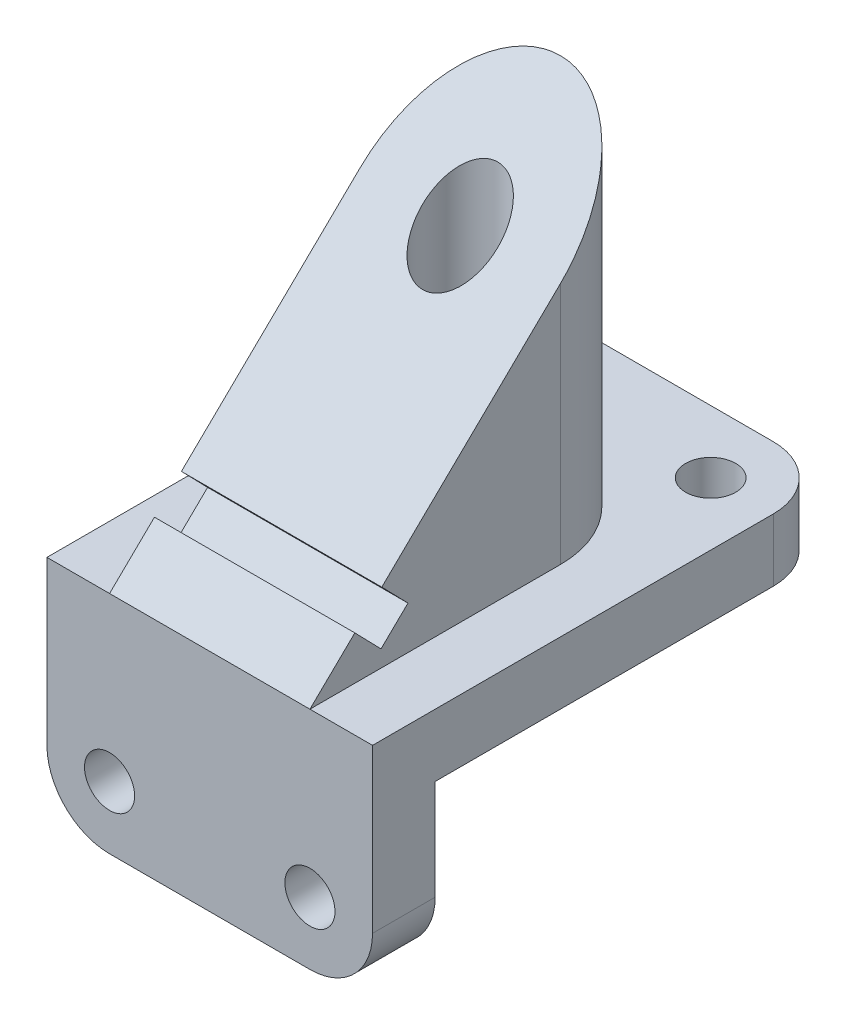
ISO-10303-21;
HEADER;
FILE_DESCRIPTION(('STEP AP214'),'2;1');
FILE_NAME('part.step','',(''),(''),'','','');
FILE_SCHEMA(('AUTOMOTIVE_DESIGN { 1 0 10303 214 1 1 1 1 }'));
ENDSEC;
DATA;
#1=APPLICATION_CONTEXT('core data for automotive mechanical design processes');
#2=APPLICATION_PROTOCOL_DEFINITION('international standard','automotive_design',2000,#1);
#3=PRODUCT_CONTEXT('',#1,'mechanical');
#4=PRODUCT('Part','Part','',(#3));
#5=PRODUCT_RELATED_PRODUCT_CATEGORY('part','',(#4));
#6=PRODUCT_DEFINITION_FORMATION('','',#4);
#7=PRODUCT_DEFINITION_CONTEXT('part definition',#1,'design');
#8=PRODUCT_DEFINITION('design','',#6,#7);
#9=PRODUCT_DEFINITION_SHAPE('','',#8);
#10=(LENGTH_UNIT() NAMED_UNIT(*) SI_UNIT(.MILLI.,.METRE.));
#11=(NAMED_UNIT(*) PLANE_ANGLE_UNIT() SI_UNIT($,.RADIAN.));
#12=(NAMED_UNIT(*) SI_UNIT($,.STERADIAN.) SOLID_ANGLE_UNIT());
#13=UNCERTAINTY_MEASURE_WITH_UNIT(LENGTH_MEASURE(1.E-05),#10,'distance_accuracy_value','');
#14=(GEOMETRIC_REPRESENTATION_CONTEXT(3) GLOBAL_UNCERTAINTY_ASSIGNED_CONTEXT((#13)) GLOBAL_UNIT_ASSIGNED_CONTEXT((#10,
#11,#12)) REPRESENTATION_CONTEXT('',''));
#15=CARTESIAN_POINT('',(0.,0.,0.));
#16=DIRECTION('',(0.,0.,1.));
#17=DIRECTION('',(1.,0.,0.));
#18=AXIS2_PLACEMENT_3D('',#15,#16,#17);
#19=CARTESIAN_POINT('',(-100.89539748954,12.4947501049979,12.1377572448551));
#20=DIRECTION('',(0.,-0.717279380859227,-0.696785684263249));
#21=DIRECTION('',(0.,0.696785684263249,-0.717279380859227));
#22=AXIS2_PLACEMENT_3D('',#19,#20,#21);
#23=PLANE('',#22);
#24=DIRECTION('',(0.,0.696785684263249,-0.717279380859227));
#25=VECTOR('',#24,1.);
#26=CARTESIAN_POINT('',(35.1046025104604,12.4947501049979,12.1377572448551));
#27=LINE('',#26,#25);
#28=CARTESIAN_POINT('',(35.1046025104604,0.,25.));
#29=VERTEX_POINT('',#28);
#30=CARTESIAN_POINT('',(35.1046025104604,17.4196421065812,7.06801547851933));
#31=VERTEX_POINT('',#30);
#32=EDGE_CURVE('E195',#29,#31,#27,.T.);
#33=ORIENTED_EDGE('',*,*,#32,.T.);
#34=DIRECTION('',(-1.,0.,0.));
#35=VECTOR('',#34,1.);
#36=CARTESIAN_POINT('',(-100.89539748954,17.4196421065812,7.06801547851933));
#37=LINE('',#36,#35);
#38=CARTESIAN_POINT('',(-44.8953974895396,17.4196421065812,7.06801547851933));
#39=VERTEX_POINT('',#38);
#40=EDGE_CURVE('E11',#31,#39,#37,.T.);
#41=ORIENTED_EDGE('',*,*,#40,.T.);
#42=DIRECTION('',(0.,0.696785684263249,-0.717279380859227));
#43=VECTOR('',#42,1.);
#44=CARTESIAN_POINT('',(-44.8953974895396,66.0293994120118,-42.9714405711886));
#45=LINE('',#44,#43);
#46=CARTESIAN_POINT('',(-44.8953974895396,0.,25.));
#47=VERTEX_POINT('',#46);
#48=EDGE_CURVE('E203',#47,#39,#45,.T.);
#49=ORIENTED_EDGE('',*,*,#48,.F.);
#50=DIRECTION('',(1.,0.,0.));
#51=VECTOR('',#50,1.);
#52=CARTESIAN_POINT('',(-100.89539748954,0.,25.));
#53=LINE('',#52,#51);
#54=EDGE_CURVE('E192',#47,#29,#53,.T.);
#55=ORIENTED_EDGE('',*,*,#54,.T.);
#56=EDGE_LOOP('',(#33,#41,#49,#55));
#57=FACE_BOUND('',#56,.T.);
#58=ADVANCED_FACE('F43',(#57),#23,.F.);
#59=CARTESIAN_POINT('',(-69.8953974895398,0.,25.));
#60=DIRECTION('',(1.,0.,0.));
#61=DIRECTION('',(0.,1.,0.));
#62=AXIS2_PLACEMENT_3D('',#59,#60,#61);
#63=PLANE('',#62);
#64=DIRECTION('',(0.,1.,0.));
#65=VECTOR('',#64,1.);
#66=CARTESIAN_POINT('',(-69.8953974895398,-160.,-135.));
#67=LINE('',#66,#65);
#68=CARTESIAN_POINT('',(-69.8953974895398,-25.,-135.));
#69=VERTEX_POINT('',#68);
#70=CARTESIAN_POINT('',(-69.8953974895398,0.,-135.));
#71=VERTEX_POINT('',#70);
#72=EDGE_CURVE('E229',#69,#71,#67,.T.);
#73=ORIENTED_EDGE('',*,*,#72,.F.);
#74=DIRECTION('',(0.,0.,1.));
#75=VECTOR('',#74,1.);
#76=CARTESIAN_POINT('',(-69.8953974895398,-25.,-160.));
#77=LINE('',#76,#75);
#78=CARTESIAN_POINT('',(-69.8953974895398,-25.,0.));
#79=VERTEX_POINT('',#78);
#80=EDGE_CURVE('E249',#69,#79,#77,.T.);
#81=ORIENTED_EDGE('',*,*,#80,.T.);
#82=DIRECTION('',(0.,-1.,0.));
#83=VECTOR('',#82,1.);
#84=CARTESIAN_POINT('',(-69.8953974895398,0.,0.));
#85=LINE('',#84,#83);
#86=CARTESIAN_POINT('',(-69.8953974895397,-64.9999999999998,0.));
#87=VERTEX_POINT('',#86);
#88=EDGE_CURVE('E268',#79,#87,#85,.T.);
#89=ORIENTED_EDGE('',*,*,#88,.T.);
#90=DIRECTION('',(0.,0.,-1.));
#91=VECTOR('',#90,1.);
#92=CARTESIAN_POINT('',(-69.8953974895397,-64.9999999999998,25.));
#93=LINE('',#92,#91);
#94=CARTESIAN_POINT('',(-69.8953974895397,-64.9999999999998,25.));
#95=VERTEX_POINT('',#94);
#96=EDGE_CURVE('E307',#95,#87,#93,.T.);
#97=ORIENTED_EDGE('',*,*,#96,.F.);
#98=DIRECTION('',(0.,-1.,0.));
#99=VECTOR('',#98,1.);
#100=CARTESIAN_POINT('',(-69.8953974895398,0.,25.));
#101=LINE('',#100,#99);
#102=CARTESIAN_POINT('',(-69.8953974895398,0.,25.));
#103=VERTEX_POINT('',#102);
#104=EDGE_CURVE('E269',#103,#95,#101,.T.);
#105=ORIENTED_EDGE('',*,*,#104,.F.);
#106=DIRECTION('',(0.,0.,-1.));
#107=VECTOR('',#106,1.);
#108=CARTESIAN_POINT('',(-69.8953974895398,0.,25.));
#109=LINE('',#108,#107);
#110=EDGE_CURVE('E284',#103,#71,#109,.T.);
#111=ORIENTED_EDGE('',*,*,#110,.T.);
#112=EDGE_LOOP('',(#73,#81,#89,#97,#105,#111));
#113=FACE_BOUND('',#112,.T.);
#114=ADVANCED_FACE('F44',(#113),#63,.F.);
#115=CARTESIAN_POINT('',(60.1046025104603,0.,25.));
#116=DIRECTION('',(-1.,0.,0.));
#117=DIRECTION('',(0.,-1.,0.));
#118=AXIS2_PLACEMENT_3D('',#115,#116,#117);
#119=PLANE('',#118);
#120=DIRECTION('',(0.,1.,0.));
#121=VECTOR('',#120,1.);
#122=CARTESIAN_POINT('',(60.1046025104603,-160.,-135.));
#123=LINE('',#122,#121);
#124=CARTESIAN_POINT('',(60.1046025104603,-25.,-135.));
#125=VERTEX_POINT('',#124);
#126=CARTESIAN_POINT('',(60.1046025104603,0.,-135.));
#127=VERTEX_POINT('',#126);
#128=EDGE_CURVE('E230',#125,#127,#123,.T.);
#129=ORIENTED_EDGE('',*,*,#128,.T.);
#130=DIRECTION('',(0.,0.,-1.));
#131=VECTOR('',#130,1.);
#132=CARTESIAN_POINT('',(60.1046025104603,0.,25.));
#133=LINE('',#132,#131);
#134=CARTESIAN_POINT('',(60.1046025104603,0.,25.));
#135=VERTEX_POINT('',#134);
#136=EDGE_CURVE('E300',#135,#127,#133,.T.);
#137=ORIENTED_EDGE('',*,*,#136,.F.);
#138=DIRECTION('',(0.,1.,0.));
#139=VECTOR('',#138,1.);
#140=CARTESIAN_POINT('',(60.1046025104603,0.,25.));
#141=LINE('',#140,#139);
#142=CARTESIAN_POINT('',(60.1046025104603,-64.9999999999998,25.));
#143=VERTEX_POINT('',#142);
#144=EDGE_CURVE('E278',#143,#135,#141,.T.);
#145=ORIENTED_EDGE('',*,*,#144,.F.);
#146=DIRECTION('',(0.,0.,-1.));
#147=VECTOR('',#146,1.);
#148=CARTESIAN_POINT('',(60.1046025104603,-64.9999999999998,25.));
#149=LINE('',#148,#147);
#150=CARTESIAN_POINT('',(60.1046025104603,-64.9999999999998,0.));
#151=VERTEX_POINT('',#150);
#152=EDGE_CURVE('E297',#143,#151,#149,.T.);
#153=ORIENTED_EDGE('',*,*,#152,.T.);
#154=DIRECTION('',(0.,1.,0.));
#155=VECTOR('',#154,1.);
#156=CARTESIAN_POINT('',(60.1046025104603,0.,0.));
#157=LINE('',#156,#155);
#158=CARTESIAN_POINT('',(60.1046025104603,-25.,0.));
#159=VERTEX_POINT('',#158);
#160=EDGE_CURVE('E271',#151,#159,#157,.T.);
#161=ORIENTED_EDGE('',*,*,#160,.T.);
#162=DIRECTION('',(0.,0.,1.));
#163=VECTOR('',#162,1.);
#164=CARTESIAN_POINT('',(60.1046025104603,-25.,-160.));
#165=LINE('',#164,#163);
#166=EDGE_CURVE('E251',#125,#159,#165,.T.);
#167=ORIENTED_EDGE('',*,*,#166,.F.);
#168=EDGE_LOOP('',(#129,#137,#145,#153,#161,#167));
#169=FACE_BOUND('',#168,.T.);
#170=ADVANCED_FACE('F358',(#169),#119,.F.);
#171=CARTESIAN_POINT('',(-69.8953974895398,0.,25.));
#172=DIRECTION('',(0.,-1.,0.));
#173=DIRECTION('',(0.,0.,-1.));
#174=AXIS2_PLACEMENT_3D('',#171,#172,#173);
#175=PLANE('',#174);
#176=DIRECTION('',(0.,0.,1.));
#177=VECTOR('',#176,1.);
#178=CARTESIAN_POINT('',(-44.8953974895396,0.,25.));
#179=LINE('',#178,#177);
#180=CARTESIAN_POINT('',(-44.8953974895396,0.,-75.));
#181=VERTEX_POINT('',#180);
#182=EDGE_CURVE('E210',#181,#47,#179,.T.);
#183=ORIENTED_EDGE('',*,*,#182,.F.);
#184=CARTESIAN_POINT('',(-4.89539748953956,0.,-75.));
#185=DIRECTION('',(0.,1.,0.));
#186=DIRECTION('',(0.,0.,-1.));
#187=AXIS2_PLACEMENT_3D('',#184,#185,#186);
#188=CIRCLE('',#187,40.);
#189=CARTESIAN_POINT('',(35.1046025104604,0.,-75.));
#190=VERTEX_POINT('',#189);
#191=EDGE_CURVE('E215',#190,#181,#188,.T.);
#192=ORIENTED_EDGE('',*,*,#191,.F.);
#193=DIRECTION('',(0.,0.,-1.));
#194=VECTOR('',#193,1.);
#195=CARTESIAN_POINT('',(35.1046025104604,0.,25.));
#196=LINE('',#195,#194);
#197=EDGE_CURVE('E208',#29,#190,#196,.T.);
#198=ORIENTED_EDGE('',*,*,#197,.F.);
#199=DIRECTION('',(-1.,0.,0.));
#200=VECTOR('',#199,1.);
#201=CARTESIAN_POINT('',(-69.8953974895398,0.,25.));
#202=LINE('',#201,#200);
#203=EDGE_CURVE('E285',#135,#29,#202,.T.);
#204=ORIENTED_EDGE('',*,*,#203,.F.);
#205=ORIENTED_EDGE('',*,*,#136,.T.);
#206=CARTESIAN_POINT('',(35.1046025104603,0.,-135.));
#207=DIRECTION('',(0.,1.,0.));
#208=DIRECTION('',(0.,0.,1.));
#209=AXIS2_PLACEMENT_3D('',#206,#207,#208);
#210=CIRCLE('',#209,25.);
#211=CARTESIAN_POINT('',(35.1046025104601,0.,-160.));
#212=VERTEX_POINT('',#211);
#213=EDGE_CURVE('E227',#212,#127,#210,.F.);
#214=ORIENTED_EDGE('',*,*,#213,.F.);
#215=DIRECTION('',(1.,0.,0.));
#216=VECTOR('',#215,1.);
#217=CARTESIAN_POINT('',(60.1046025104603,0.,-160.));
#218=LINE('',#217,#216);
#219=CARTESIAN_POINT('',(-44.8953974895396,0.,-160.));
#220=VERTEX_POINT('',#219);
#221=EDGE_CURVE('E250',#220,#212,#218,.T.);
#222=ORIENTED_EDGE('',*,*,#221,.F.);
#223=CARTESIAN_POINT('',(-44.8953974895398,0.,-135.));
#224=DIRECTION('',(0.,1.,0.));
#225=DIRECTION('',(0.,0.,1.));
#226=AXIS2_PLACEMENT_3D('',#223,#224,#225);
#227=CIRCLE('',#226,25.);
#228=EDGE_CURVE('E234',#220,#71,#227,.T.);
#229=ORIENTED_EDGE('',*,*,#228,.T.);
#230=ORIENTED_EDGE('',*,*,#110,.F.);
#231=EDGE_CURVE('E281',#47,#103,#202,.T.);
#232=ORIENTED_EDGE('',*,*,#231,.F.);
#233=EDGE_LOOP('',(#183,#192,#198,#204,#205,#214,#222,#229,#230,#232));
#234=FACE_BOUND('',#233,.T.);
#235=CARTESIAN_POINT('',(-44.8953974895398,0.,-135.));
#236=DIRECTION('',(0.,1.,0.));
#237=DIRECTION('',(0.,0.,1.));
#238=AXIS2_PLACEMENT_3D('',#235,#236,#237);
#239=CIRCLE('',#238,10.);
#240=CARTESIAN_POINT('',(-44.8953974895398,0.,-125.));
#241=VERTEX_POINT('',#240);
#242=EDGE_CURVE('E223',#241,#241,#239,.T.);
#243=ORIENTED_EDGE('',*,*,#242,.F.);
#244=EDGE_LOOP('',(#243));
#245=FACE_BOUND('',#244,.T.);
#246=CARTESIAN_POINT('',(35.1046025104603,0.,-135.));
#247=DIRECTION('',(0.,1.,0.));
#248=DIRECTION('',(0.,0.,1.));
#249=AXIS2_PLACEMENT_3D('',#246,#247,#248);
#250=CIRCLE('',#249,10.);
#251=CARTESIAN_POINT('',(35.1046025104603,0.,-125.));
#252=VERTEX_POINT('',#251);
#253=EDGE_CURVE('E219',#252,#252,#250,.T.);
#254=ORIENTED_EDGE('',*,*,#253,.F.);
#255=EDGE_LOOP('',(#254));
#256=FACE_BOUND('',#255,.T.);
#257=ADVANCED_FACE('F331',(#234,#245,#256),#175,.F.);
#258=CARTESIAN_POINT('',(60.1046025104603,-25.,-160.));
#259=DIRECTION('',(0.,1.,0.));
#260=DIRECTION('',(0.,0.,1.));
#261=AXIS2_PLACEMENT_3D('',#258,#259,#260);
#262=PLANE('',#261);
#263=CARTESIAN_POINT('',(-44.8953974895398,-25.,-135.));
#264=DIRECTION('',(0.,1.,0.));
#265=DIRECTION('',(0.,0.,1.));
#266=AXIS2_PLACEMENT_3D('',#263,#264,#265);
#267=CIRCLE('',#266,10.);
#268=CARTESIAN_POINT('',(-44.8953974895398,-25.,-125.));
#269=VERTEX_POINT('',#268);
#270=EDGE_CURVE('E240',#269,#269,#267,.T.);
#271=ORIENTED_EDGE('',*,*,#270,.T.);
#272=EDGE_LOOP('',(#271));
#273=FACE_BOUND('',#272,.T.);
#274=CARTESIAN_POINT('',(35.1046025104603,-25.,-135.));
#275=DIRECTION('',(0.,1.,0.));
#276=DIRECTION('',(0.,0.,1.));
#277=AXIS2_PLACEMENT_3D('',#274,#275,#276);
#278=CIRCLE('',#277,10.);
#279=CARTESIAN_POINT('',(35.1046025104603,-25.,-125.));
#280=VERTEX_POINT('',#279);
#281=EDGE_CURVE('E224',#280,#280,#278,.T.);
#282=ORIENTED_EDGE('',*,*,#281,.T.);
#283=EDGE_LOOP('',(#282));
#284=FACE_BOUND('',#283,.T.);
#285=DIRECTION('',(-1.,0.,0.));
#286=VECTOR('',#285,1.);
#287=CARTESIAN_POINT('',(60.1046025104603,-25.,-160.));
#288=LINE('',#287,#286);
#289=CARTESIAN_POINT('',(35.1046025104603,-25.,-160.));
#290=VERTEX_POINT('',#289);
#291=CARTESIAN_POINT('',(-44.8953974895396,-25.,-160.));
#292=VERTEX_POINT('',#291);
#293=EDGE_CURVE('E242',#290,#292,#288,.T.);
#294=ORIENTED_EDGE('',*,*,#293,.F.);
#295=CARTESIAN_POINT('',(35.1046025104603,-25.,-135.));
#296=DIRECTION('',(0.,1.,0.));
#297=DIRECTION('',(0.,0.,1.));
#298=AXIS2_PLACEMENT_3D('',#295,#296,#297);
#299=CIRCLE('',#298,25.);
#300=EDGE_CURVE('E239',#290,#125,#299,.F.);
#301=ORIENTED_EDGE('',*,*,#300,.T.);
#302=ORIENTED_EDGE('',*,*,#166,.T.);
#303=DIRECTION('',(-1.,0.,0.));
#304=VECTOR('',#303,1.);
#305=CARTESIAN_POINT('',(60.1046025104603,-25.,0.));
#306=LINE('',#305,#304);
#307=EDGE_CURVE('E243',#159,#79,#306,.T.);
#308=ORIENTED_EDGE('',*,*,#307,.T.);
#309=ORIENTED_EDGE('',*,*,#80,.F.);
#310=CARTESIAN_POINT('',(-44.8953974895398,-25.,-135.));
#311=DIRECTION('',(0.,1.,0.));
#312=DIRECTION('',(0.,0.,1.));
#313=AXIS2_PLACEMENT_3D('',#310,#311,#312);
#314=CIRCLE('',#313,25.);
#315=EDGE_CURVE('E231',#292,#69,#314,.T.);
#316=ORIENTED_EDGE('',*,*,#315,.F.);
#317=EDGE_LOOP('',(#294,#301,#302,#308,#309,#316));
#318=FACE_BOUND('',#317,.T.);
#319=ADVANCED_FACE('F405',(#273,#284,#318),#262,.F.);
#320=CARTESIAN_POINT('',(0.,0.,-160.));
#321=DIRECTION('',(0.,0.,-1.));
#322=DIRECTION('',(-1.,0.,0.));
#323=AXIS2_PLACEMENT_3D('',#320,#321,#322);
#324=PLANE('',#323);
#325=ORIENTED_EDGE('',*,*,#221,.T.);
#326=DIRECTION('',(0.,1.,0.));
#327=VECTOR('',#326,1.);
#328=CARTESIAN_POINT('',(35.1046025104603,-160.,-160.));
#329=LINE('',#328,#327);
#330=EDGE_CURVE('E314',#212,#290,#329,.F.);
#331=ORIENTED_EDGE('',*,*,#330,.T.);
#332=ORIENTED_EDGE('',*,*,#293,.T.);
#333=DIRECTION('',(0.,1.,0.));
#334=VECTOR('',#333,1.);
#335=CARTESIAN_POINT('',(-44.8953974895398,-160.,-160.));
#336=LINE('',#335,#334);
#337=EDGE_CURVE('E315',#292,#220,#336,.T.);
#338=ORIENTED_EDGE('',*,*,#337,.T.);
#339=EDGE_LOOP('',(#325,#331,#332,#338));
#340=FACE_BOUND('',#339,.T.);
#341=ADVANCED_FACE('F396',(#340),#324,.T.);
#342=CARTESIAN_POINT('',(-44.8953974895397,-65.,0.));
#343=DIRECTION('',(0.,0.,1.));
#344=DIRECTION('',(1.,0.,0.));
#345=AXIS2_PLACEMENT_3D('',#342,#343,#344);
#346=PLANE('',#345);
#347=CARTESIAN_POINT('',(35.1046025104603,-65.,0.));
#348=DIRECTION('',(0.,0.,1.));
#349=DIRECTION('',(1.,0.,0.));
#350=AXIS2_PLACEMENT_3D('',#347,#348,#349);
#351=CIRCLE('',#350,10.);
#352=CARTESIAN_POINT('',(45.1046025104603,-65.,0.));
#353=VERTEX_POINT('',#352);
#354=EDGE_CURVE('E259',#353,#353,#351,.T.);
#355=ORIENTED_EDGE('',*,*,#354,.T.);
#356=EDGE_LOOP('',(#355));
#357=FACE_BOUND('',#356,.T.);
#358=CARTESIAN_POINT('',(-44.8953974895397,-65.,0.));
#359=DIRECTION('',(0.,0.,1.));
#360=DIRECTION('',(1.,0.,0.));
#361=AXIS2_PLACEMENT_3D('',#358,#359,#360);
#362=CIRCLE('',#361,10.);
#363=CARTESIAN_POINT('',(-34.8953974895397,-65.,0.));
#364=VERTEX_POINT('',#363);
#365=EDGE_CURVE('E257',#364,#364,#362,.T.);
#366=ORIENTED_EDGE('',*,*,#365,.T.);
#367=EDGE_LOOP('',(#366));
#368=FACE_BOUND('',#367,.T.);
#369=ORIENTED_EDGE('',*,*,#307,.F.);
#370=ORIENTED_EDGE('',*,*,#160,.F.);
#371=CARTESIAN_POINT('',(35.1046025104603,-65.,0.));
#372=DIRECTION('',(0.,0.,1.));
#373=DIRECTION('',(1.,0.,0.));
#374=AXIS2_PLACEMENT_3D('',#371,#372,#373);
#375=CIRCLE('',#374,25.);
#376=CARTESIAN_POINT('',(35.1046025104601,-90.,0.));
#377=VERTEX_POINT('',#376);
#378=EDGE_CURVE('E293',#377,#151,#375,.T.);
#379=ORIENTED_EDGE('',*,*,#378,.F.);
#380=DIRECTION('',(1.,0.,0.));
#381=VECTOR('',#380,1.);
#382=CARTESIAN_POINT('',(-44.8953974895396,-90.,0.));
#383=LINE('',#382,#381);
#384=CARTESIAN_POINT('',(-44.8953974895396,-90.,0.));
#385=VERTEX_POINT('',#384);
#386=EDGE_CURVE('E289',#385,#377,#383,.T.);
#387=ORIENTED_EDGE('',*,*,#386,.F.);
#388=CARTESIAN_POINT('',(-44.8953974895397,-65.,0.));
#389=DIRECTION('',(0.,0.,1.));
#390=DIRECTION('',(1.,0.,0.));
#391=AXIS2_PLACEMENT_3D('',#388,#389,#390);
#392=CIRCLE('',#391,25.);
#393=EDGE_CURVE('E290',#87,#385,#392,.T.);
#394=ORIENTED_EDGE('',*,*,#393,.F.);
#395=ORIENTED_EDGE('',*,*,#88,.F.);
#396=EDGE_LOOP('',(#369,#370,#379,#387,#394,#395));
#397=FACE_BOUND('',#396,.T.);
#398=ADVANCED_FACE('F402',(#357,#368,#397),#346,.F.);
#399=CARTESIAN_POINT('',(-44.8953974895397,-65.,25.));
#400=DIRECTION('',(0.,0.,1.));
#401=DIRECTION('',(1.,0.,0.));
#402=AXIS2_PLACEMENT_3D('',#399,#400,#401);
#403=PLANE('',#402);
#404=ORIENTED_EDGE('',*,*,#54,.F.);
#405=ORIENTED_EDGE('',*,*,#231,.T.);
#406=ORIENTED_EDGE('',*,*,#104,.T.);
#407=CARTESIAN_POINT('',(-44.8953974895397,-65.,25.));
#408=DIRECTION('',(0.,0.,1.));
#409=DIRECTION('',(1.,0.,0.));
#410=AXIS2_PLACEMENT_3D('',#407,#408,#409);
#411=CIRCLE('',#410,25.);
#412=CARTESIAN_POINT('',(-44.8953974895396,-90.,25.));
#413=VERTEX_POINT('',#412);
#414=EDGE_CURVE('E275',#95,#413,#411,.T.);
#415=ORIENTED_EDGE('',*,*,#414,.T.);
#416=DIRECTION('',(1.,0.,0.));
#417=VECTOR('',#416,1.);
#418=CARTESIAN_POINT('',(-44.8953974895396,-90.,25.));
#419=LINE('',#418,#417);
#420=CARTESIAN_POINT('',(35.1046025104601,-90.,25.));
#421=VERTEX_POINT('',#420);
#422=EDGE_CURVE('E273',#413,#421,#419,.T.);
#423=ORIENTED_EDGE('',*,*,#422,.T.);
#424=CARTESIAN_POINT('',(35.1046025104603,-65.,25.));
#425=DIRECTION('',(0.,0.,1.));
#426=DIRECTION('',(1.,0.,0.));
#427=AXIS2_PLACEMENT_3D('',#424,#425,#426);
#428=CIRCLE('',#427,25.);
#429=EDGE_CURVE('E276',#421,#143,#428,.T.);
#430=ORIENTED_EDGE('',*,*,#429,.T.);
#431=ORIENTED_EDGE('',*,*,#144,.T.);
#432=ORIENTED_EDGE('',*,*,#203,.T.);
#433=EDGE_LOOP('',(#404,#405,#406,#415,#423,#430,#431,#432));
#434=FACE_BOUND('',#433,.T.);
#435=CARTESIAN_POINT('',(-44.8953974895397,-65.,25.));
#436=DIRECTION('',(0.,0.,1.));
#437=DIRECTION('',(1.,0.,0.));
#438=AXIS2_PLACEMENT_3D('',#435,#436,#437);
#439=CIRCLE('',#438,10.);
#440=CARTESIAN_POINT('',(-34.8953974895397,-65.,25.));
#441=VERTEX_POINT('',#440);
#442=EDGE_CURVE('E263',#441,#441,#439,.T.);
#443=ORIENTED_EDGE('',*,*,#442,.F.);
#444=EDGE_LOOP('',(#443));
#445=FACE_BOUND('',#444,.T.);
#446=CARTESIAN_POINT('',(35.1046025104603,-65.,25.));
#447=DIRECTION('',(0.,0.,1.));
#448=DIRECTION('',(1.,0.,0.));
#449=AXIS2_PLACEMENT_3D('',#446,#447,#448);
#450=CIRCLE('',#449,10.);
#451=CARTESIAN_POINT('',(45.1046025104603,-65.,25.));
#452=VERTEX_POINT('',#451);
#453=EDGE_CURVE('E256',#452,#452,#450,.T.);
#454=ORIENTED_EDGE('',*,*,#453,.F.);
#455=EDGE_LOOP('',(#454));
#456=FACE_BOUND('',#455,.T.);
#457=ADVANCED_FACE('F414',(#434,#445,#456),#403,.T.);
#458=CARTESIAN_POINT('',(-44.8953974895397,-65.,25.));
#459=DIRECTION('',(0.,0.,-1.));
#460=DIRECTION('',(-1.,0.,0.));
#461=AXIS2_PLACEMENT_3D('',#458,#459,#460);
#462=CYLINDRICAL_SURFACE('',#461,25.);
#463=ORIENTED_EDGE('',*,*,#393,.T.);
#464=DIRECTION('',(0.,0.,-1.));
#465=VECTOR('',#464,1.);
#466=CARTESIAN_POINT('',(-44.8953974895396,-90.,25.));
#467=LINE('',#466,#465);
#468=EDGE_CURVE('E306',#413,#385,#467,.T.);
#469=ORIENTED_EDGE('',*,*,#468,.F.);
#470=ORIENTED_EDGE('',*,*,#414,.F.);
#471=ORIENTED_EDGE('',*,*,#96,.T.);
#472=EDGE_LOOP('',(#463,#469,#470,#471));
#473=FACE_BOUND('',#472,.T.);
#474=ADVANCED_FACE('F416',(#473),#462,.T.);
#475=CARTESIAN_POINT('',(-44.8953974895396,-90.,25.));
#476=DIRECTION('',(0.,1.,0.));
#477=DIRECTION('',(0.,0.,1.));
#478=AXIS2_PLACEMENT_3D('',#475,#476,#477);
#479=PLANE('',#478);
#480=ORIENTED_EDGE('',*,*,#386,.T.);
#481=DIRECTION('',(0.,0.,-1.));
#482=VECTOR('',#481,1.);
#483=CARTESIAN_POINT('',(35.1046025104601,-90.,25.));
#484=LINE('',#483,#482);
#485=EDGE_CURVE('E303',#421,#377,#484,.T.);
#486=ORIENTED_EDGE('',*,*,#485,.F.);
#487=ORIENTED_EDGE('',*,*,#422,.F.);
#488=ORIENTED_EDGE('',*,*,#468,.T.);
#489=EDGE_LOOP('',(#480,#486,#487,#488));
#490=FACE_BOUND('',#489,.T.);
#491=ADVANCED_FACE('F429',(#490),#479,.F.);
#492=CARTESIAN_POINT('',(35.1046025104603,-65.,25.));
#493=DIRECTION('',(0.,0.,-1.));
#494=DIRECTION('',(-1.,0.,0.));
#495=AXIS2_PLACEMENT_3D('',#492,#493,#494);
#496=CYLINDRICAL_SURFACE('',#495,25.);
#497=ORIENTED_EDGE('',*,*,#378,.T.);
#498=ORIENTED_EDGE('',*,*,#152,.F.);
#499=ORIENTED_EDGE('',*,*,#429,.F.);
#500=ORIENTED_EDGE('',*,*,#485,.T.);
#501=EDGE_LOOP('',(#497,#498,#499,#500));
#502=FACE_BOUND('',#501,.T.);
#503=ADVANCED_FACE('F413',(#502),#496,.T.);
#504=CARTESIAN_POINT('',(-44.8953974895397,-65.,25.));
#505=DIRECTION('',(0.,0.,-1.));
#506=DIRECTION('',(-1.,0.,0.));
#507=AXIS2_PLACEMENT_3D('',#504,#505,#506);
#508=CYLINDRICAL_SURFACE('',#507,10.);
#509=ORIENTED_EDGE('',*,*,#442,.T.);
#510=EDGE_LOOP('',(#509));
#511=FACE_BOUND('',#510,.T.);
#512=ORIENTED_EDGE('',*,*,#365,.F.);
#513=EDGE_LOOP('',(#512));
#514=FACE_BOUND('',#513,.T.);
#515=ADVANCED_FACE('F408',(#511,#514),#508,.F.);
#516=CARTESIAN_POINT('',(35.1046025104603,-65.,25.));
#517=DIRECTION('',(0.,0.,-1.));
#518=DIRECTION('',(-1.,0.,0.));
#519=AXIS2_PLACEMENT_3D('',#516,#517,#518);
#520=CYLINDRICAL_SURFACE('',#519,10.);
#521=ORIENTED_EDGE('',*,*,#453,.T.);
#522=EDGE_LOOP('',(#521));
#523=FACE_BOUND('',#522,.T.);
#524=ORIENTED_EDGE('',*,*,#354,.F.);
#525=EDGE_LOOP('',(#524));
#526=FACE_BOUND('',#525,.T.);
#527=ADVANCED_FACE('F398',(#523,#526),#520,.F.);
#528=CARTESIAN_POINT('',(-44.8953974895398,-160.,-135.));
#529=DIRECTION('',(0.,1.,0.));
#530=DIRECTION('',(0.,0.,1.));
#531=AXIS2_PLACEMENT_3D('',#528,#529,#530);
#532=CYLINDRICAL_SURFACE('',#531,25.);
#533=ORIENTED_EDGE('',*,*,#315,.T.);
#534=ORIENTED_EDGE('',*,*,#72,.T.);
#535=ORIENTED_EDGE('',*,*,#228,.F.);
#536=ORIENTED_EDGE('',*,*,#337,.F.);
#537=EDGE_LOOP('',(#533,#534,#535,#536));
#538=FACE_BOUND('',#537,.T.);
#539=ADVANCED_FACE('F395',(#538),#532,.T.);
#540=CARTESIAN_POINT('',(35.1046025104603,-160.,-135.));
#541=DIRECTION('',(0.,1.,0.));
#542=DIRECTION('',(0.,0.,1.));
#543=AXIS2_PLACEMENT_3D('',#540,#541,#542);
#544=CYLINDRICAL_SURFACE('',#543,25.);
#545=ORIENTED_EDGE('',*,*,#330,.F.);
#546=ORIENTED_EDGE('',*,*,#213,.T.);
#547=ORIENTED_EDGE('',*,*,#128,.F.);
#548=ORIENTED_EDGE('',*,*,#300,.F.);
#549=EDGE_LOOP('',(#545,#546,#547,#548));
#550=FACE_BOUND('',#549,.T.);
#551=ADVANCED_FACE('F390',(#550),#544,.T.);
#552=CARTESIAN_POINT('',(35.1046025104603,-160.,-135.));
#553=DIRECTION('',(0.,1.,0.));
#554=DIRECTION('',(0.,0.,1.));
#555=AXIS2_PLACEMENT_3D('',#552,#553,#554);
#556=CYLINDRICAL_SURFACE('',#555,10.);
#557=ORIENTED_EDGE('',*,*,#253,.T.);
#558=EDGE_LOOP('',(#557));
#559=FACE_BOUND('',#558,.T.);
#560=ORIENTED_EDGE('',*,*,#281,.F.);
#561=EDGE_LOOP('',(#560));
#562=FACE_BOUND('',#561,.T.);
#563=ADVANCED_FACE('F381',(#559,#562),#556,.F.);
#564=CARTESIAN_POINT('',(-44.8953974895398,-160.,-135.));
#565=DIRECTION('',(0.,1.,0.));
#566=DIRECTION('',(0.,0.,1.));
#567=AXIS2_PLACEMENT_3D('',#564,#565,#566);
#568=CYLINDRICAL_SURFACE('',#567,10.);
#569=ORIENTED_EDGE('',*,*,#242,.T.);
#570=EDGE_LOOP('',(#569));
#571=FACE_BOUND('',#570,.T.);
#572=ORIENTED_EDGE('',*,*,#270,.F.);
#573=EDGE_LOOP('',(#572));
#574=FACE_BOUND('',#573,.T.);
#575=ADVANCED_FACE('F382',(#571,#574),#568,.F.);
#576=CARTESIAN_POINT('',(-44.8953974895396,136.,25.));
#577=DIRECTION('',(1.,0.,0.));
#578=DIRECTION('',(0.,0.,-1.));
#579=AXIS2_PLACEMENT_3D('',#576,#577,#578);
#580=PLANE('',#579);
#581=ORIENTED_EDGE('',*,*,#48,.T.);
#582=DIRECTION('',(0.,-0.717279380859227,-0.696785684263249));
#583=VECTOR('',#582,1.);
#584=CARTESIAN_POINT('',(-44.8953974895396,87.3902426945695,75.0394560497079));
#585=LINE('',#584,#583);
#586=CARTESIAN_POINT('',(-44.8953974895396,6.66045139369282,-3.38376978542941));
#587=VERTEX_POINT('',#586);
#588=EDGE_CURVE('E188',#39,#587,#585,.T.);
#589=ORIENTED_EDGE('',*,*,#588,.T.);
#590=DIRECTION('',(0.,0.69678568426325,-0.717279380859226));
#591=VECTOR('',#590,1.);
#592=CARTESIAN_POINT('',(-44.8953974895396,55.2702086991235,-53.4232258351373));
#593=LINE('',#592,#591);
#594=CARTESIAN_POINT('',(-44.8953974895396,17.1122366576416,-14.1429604983178));
#595=VERTEX_POINT('',#594);
#596=EDGE_CURVE('E167',#587,#595,#593,.T.);
#597=ORIENTED_EDGE('',*,*,#596,.T.);
#598=DIRECTION('',(0.,0.717279380859227,0.696785684263249));
#599=VECTOR('',#598,1.);
#600=CARTESIAN_POINT('',(-44.8953974895396,97.8420279585182,64.2802653368195));
#601=LINE('',#600,#599);
#602=CARTESIAN_POINT('',(-44.8953974895396,27.87142737053,-3.69117523436907));
#603=VERTEX_POINT('',#602);
#604=EDGE_CURVE('E187',#595,#603,#601,.T.);
#605=ORIENTED_EDGE('',*,*,#604,.T.);
#606=CARTESIAN_POINT('',(-44.8953974895396,97.1428571428571,-75.));
#607=VERTEX_POINT('',#606);
#608=EDGE_CURVE('E199',#603,#607,#45,.T.);
#609=ORIENTED_EDGE('',*,*,#608,.T.);
#610=DIRECTION('',(0.,-1.,0.));
#611=VECTOR('',#610,1.);
#612=CARTESIAN_POINT('',(-44.8953974895396,136.,-75.));
#613=LINE('',#612,#611);
#614=EDGE_CURVE('E216',#607,#181,#613,.T.);
#615=ORIENTED_EDGE('',*,*,#614,.T.);
#616=ORIENTED_EDGE('',*,*,#182,.T.);
#617=EDGE_LOOP('',(#581,#589,#597,#605,#609,#615,#616));
#618=FACE_BOUND('',#617,.T.);
#619=ADVANCED_FACE('F339',(#618),#580,.F.);
#620=CARTESIAN_POINT('',(35.1046025104604,136.,25.));
#621=DIRECTION('',(-1.,0.,0.));
#622=DIRECTION('',(0.,0.,1.));
#623=AXIS2_PLACEMENT_3D('',#620,#621,#622);
#624=PLANE('',#623);
#625=DIRECTION('',(0.,0.696785684263249,-0.717279380859226));
#626=VECTOR('',#625,1.);
#627=CARTESIAN_POINT('',(35.1046025104604,6.66045139369282,-3.38376978542941));
#628=LINE('',#627,#626);
#629=CARTESIAN_POINT('',(35.1046025104604,6.66045139369282,-3.38376978542941));
#630=VERTEX_POINT('',#629);
#631=CARTESIAN_POINT('',(35.1046025104604,17.1122366576416,-14.1429604983178));
#632=VERTEX_POINT('',#631);
#633=EDGE_CURVE('E166',#630,#632,#628,.T.);
#634=ORIENTED_EDGE('',*,*,#633,.F.);
#635=DIRECTION('',(0.,-0.717279380859227,-0.696785684263249));
#636=VECTOR('',#635,1.);
#637=CARTESIAN_POINT('',(35.1046025104604,17.4196421065812,7.06801547851933));
#638=LINE('',#637,#636);
#639=EDGE_CURVE('E176',#31,#630,#638,.T.);
#640=ORIENTED_EDGE('',*,*,#639,.F.);
#641=ORIENTED_EDGE('',*,*,#32,.F.);
#642=ORIENTED_EDGE('',*,*,#197,.T.);
#643=DIRECTION('',(0.,-1.,0.));
#644=VECTOR('',#643,1.);
#645=CARTESIAN_POINT('',(35.1046025104604,136.,-75.));
#646=LINE('',#645,#644);
#647=CARTESIAN_POINT('',(35.1046025104604,97.1428571428572,-75.));
#648=VERTEX_POINT('',#647);
#649=EDGE_CURVE('E218',#648,#190,#646,.T.);
#650=ORIENTED_EDGE('',*,*,#649,.F.);
#651=CARTESIAN_POINT('',(35.1046025104604,27.87142737053,-3.69117523436908));
#652=VERTEX_POINT('',#651);
#653=EDGE_CURVE('E62',#652,#648,#27,.T.);
#654=ORIENTED_EDGE('',*,*,#653,.F.);
#655=DIRECTION('',(0.,0.717279380859227,0.696785684263249));
#656=VECTOR('',#655,1.);
#657=CARTESIAN_POINT('',(35.1046025104604,27.87142737053,-3.69117523436907));
#658=LINE('',#657,#656);
#659=EDGE_CURVE('E59',#632,#652,#658,.T.);
#660=ORIENTED_EDGE('',*,*,#659,.F.);
#661=EDGE_LOOP('',(#634,#640,#641,#642,#650,#654,#660));
#662=FACE_BOUND('',#661,.T.);
#663=ADVANCED_FACE('F185',(#662),#624,.F.);
#664=CARTESIAN_POINT('',(-4.89539748953956,136.,-75.));
#665=DIRECTION('',(0.,-1.,0.));
#666=DIRECTION('',(0.,0.,-1.));
#667=AXIS2_PLACEMENT_3D('',#664,#665,#666);
#668=CYLINDRICAL_SURFACE('',#667,40.);
#669=ORIENTED_EDGE('',*,*,#614,.F.);
#670=CARTESIAN_POINT('',(-4.89539748953956,97.1428571428572,-75.));
#671=DIRECTION('',(0.,-0.717279380859227,-0.696785684263249));
#672=DIRECTION('',(0.,-0.696785684263249,0.717279380859227));
#673=AXIS2_PLACEMENT_3D('',#670,#671,#672);
#674=ELLIPSE('',#673,55.7662761085982,40.);
#675=EDGE_CURVE('E198',#607,#648,#674,.T.);
#676=ORIENTED_EDGE('',*,*,#675,.T.);
#677=ORIENTED_EDGE('',*,*,#649,.T.);
#678=ORIENTED_EDGE('',*,*,#191,.T.);
#679=EDGE_LOOP('',(#669,#676,#677,#678));
#680=FACE_BOUND('',#679,.T.);
#681=ADVANCED_FACE('F329',(#680),#668,.T.);
#682=CARTESIAN_POINT('',(-4.89539748953956,97.1428571428572,-75.));
#683=DIRECTION('',(0.,-0.717279380859227,-0.696785684263249));
#684=DIRECTION('',(0.,-0.696785684263249,0.717279380859227));
#685=AXIS2_PLACEMENT_3D('',#682,#683,#684);
#686=ELLIPSE('',#685,20.9123535407243,15.);
#687=CARTESIAN_POINT('',(-4.89539748953956,82.5714285714286,-60.));
#688=VERTEX_POINT('',#687);
#689=EDGE_CURVE('E200',#688,#688,#686,.T.);
#690=ORIENTED_EDGE('',*,*,#689,.T.);
#691=EDGE_LOOP('',(#690));
#692=FACE_BOUND('',#691,.T.);
#693=ORIENTED_EDGE('',*,*,#608,.F.);
#694=DIRECTION('',(1.,0.,0.));
#695=VECTOR('',#694,1.);
#696=CARTESIAN_POINT('',(-100.89539748954,27.87142737053,-3.69117523436907));
#697=LINE('',#696,#695);
#698=EDGE_CURVE('E51',#603,#652,#697,.T.);
#699=ORIENTED_EDGE('',*,*,#698,.T.);
#700=ORIENTED_EDGE('',*,*,#653,.T.);
#701=ORIENTED_EDGE('',*,*,#675,.F.);
#702=EDGE_LOOP('',(#693,#699,#700,#701));
#703=FACE_BOUND('',#702,.T.);
#704=ADVANCED_FACE('F323',(#692,#703),#23,.F.);
#705=CARTESIAN_POINT('',(-4.89539748953956,0.,-75.));
#706=DIRECTION('',(0.,1.,0.));
#707=DIRECTION('',(0.,0.,1.));
#708=AXIS2_PLACEMENT_3D('',#705,#706,#707);
#709=CIRCLE('',#708,15.);
#710=CARTESIAN_POINT('',(-4.89539748953956,0.,-60.));
#711=VERTEX_POINT('',#710);
#712=EDGE_CURVE('E204',#711,#711,#709,.T.);
#713=ORIENTED_EDGE('',*,*,#712,.T.);
#714=EDGE_LOOP('',(#713));
#715=FACE_BOUND('',#714,.T.);
#716=ADVANCED_FACE('F359',(#715),#175,.F.);
#717=CARTESIAN_POINT('',(-4.89539748953956,136.,-75.));
#718=DIRECTION('',(0.,-1.,0.));
#719=DIRECTION('',(0.,0.,-1.));
#720=AXIS2_PLACEMENT_3D('',#717,#718,#719);
#721=CYLINDRICAL_SURFACE('',#720,15.);
#722=ORIENTED_EDGE('',*,*,#689,.F.);
#723=EDGE_LOOP('',(#722));
#724=FACE_BOUND('',#723,.T.);
#725=ORIENTED_EDGE('',*,*,#712,.F.);
#726=EDGE_LOOP('',(#725));
#727=FACE_BOUND('',#726,.T.);
#728=ADVANCED_FACE('F370',(#724,#727),#721,.F.);
#729=CARTESIAN_POINT('',(-100.89539748954,6.66045139369282,-3.38376978542941));
#730=DIRECTION('',(0.,-0.717279380859226,-0.69678568426325));
#731=DIRECTION('',(0.,0.69678568426325,-0.717279380859226));
#732=AXIS2_PLACEMENT_3D('',#729,#730,#731);
#733=PLANE('',#732);
#734=DIRECTION('',(1.,0.,0.));
#735=VECTOR('',#734,1.);
#736=CARTESIAN_POINT('',(-100.89539748954,6.66045139369282,-3.38376978542941));
#737=LINE('',#736,#735);
#738=EDGE_CURVE('E161',#587,#630,#737,.T.);
#739=ORIENTED_EDGE('',*,*,#738,.T.);
#740=ORIENTED_EDGE('',*,*,#633,.T.);
#741=DIRECTION('',(1.,0.,0.));
#742=VECTOR('',#741,1.);
#743=CARTESIAN_POINT('',(-100.89539748954,17.1122366576416,-14.1429604983178));
#744=LINE('',#743,#742);
#745=EDGE_CURVE('E173',#595,#632,#744,.T.);
#746=ORIENTED_EDGE('',*,*,#745,.F.);
#747=ORIENTED_EDGE('',*,*,#596,.F.);
#748=EDGE_LOOP('',(#739,#740,#746,#747));
#749=FACE_BOUND('',#748,.T.);
#750=ADVANCED_FACE('F164',(#749),#733,.F.);
#751=CARTESIAN_POINT('',(-100.89539748954,17.4196421065812,7.06801547851933));
#752=DIRECTION('',(0.,-0.696785684263249,0.717279380859227));
#753=DIRECTION('',(0.,-0.717279380859227,-0.696785684263249));
#754=AXIS2_PLACEMENT_3D('',#751,#752,#753);
#755=PLANE('',#754);
#756=ORIENTED_EDGE('',*,*,#40,.F.);
#757=ORIENTED_EDGE('',*,*,#639,.T.);
#758=ORIENTED_EDGE('',*,*,#738,.F.);
#759=ORIENTED_EDGE('',*,*,#588,.F.);
#760=EDGE_LOOP('',(#756,#757,#758,#759));
#761=FACE_BOUND('',#760,.T.);
#762=ADVANCED_FACE('F180',(#761),#755,.F.);
#763=CARTESIAN_POINT('',(-100.89539748954,27.87142737053,-3.69117523436907));
#764=DIRECTION('',(0.,0.696785684263249,-0.717279380859227));
#765=DIRECTION('',(0.,0.717279380859227,0.696785684263249));
#766=AXIS2_PLACEMENT_3D('',#763,#764,#765);
#767=PLANE('',#766);
#768=ORIENTED_EDGE('',*,*,#745,.T.);
#769=ORIENTED_EDGE('',*,*,#659,.T.);
#770=ORIENTED_EDGE('',*,*,#698,.F.);
#771=ORIENTED_EDGE('',*,*,#604,.F.);
#772=EDGE_LOOP('',(#768,#769,#770,#771));
#773=FACE_BOUND('',#772,.T.);
#774=ADVANCED_FACE('F338',(#773),#767,.F.);
#775=CLOSED_SHELL('',(#58,#114,#170,#257,#319,#341,#398,#457,#474,#491,#503,#515,#527,#539,#551,
#563,#575,#619,#663,#681,#704,#716,#728,#750,#762,#774));
#776=MANIFOLD_SOLID_BREP('B2',#775);
#777=ADVANCED_BREP_SHAPE_REPRESENTATION('',(#18,#776),#14);
#778=SHAPE_DEFINITION_REPRESENTATION(#9,#777);
ENDSEC;
END-ISO-10303-21;
